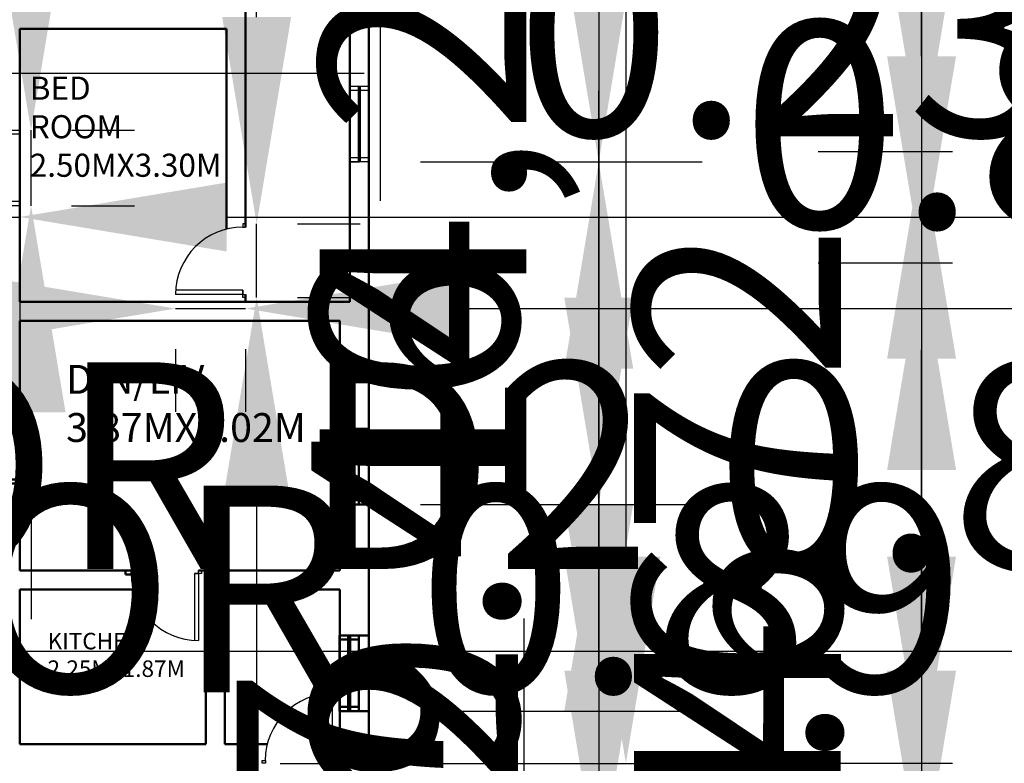
# Model space of a CAD drawing. Units: metres. Extents: x 782 to 1487, y 1262 to 7446.
# Tile 14 of 25: x 828 to 840, y 1293 to 1302. Entities that reach past the tile are written whole.
import ezdxf

# ---------------------------------------------------------------- set-up
doc = ezdxf.new("R2010")
doc.units = ezdxf.units.M
for name, color, linetype, lineweight in [('A-ANNO-DIMS', 2, 'Continuous', 18), ('A-AREA-IDEN', 3, 'Continuous', 18), ('A-DOOR', 4, 'Continuous', 25), ('A-GLAZ', 4, 'Continuous', 25), ('A-WALL', 7, 'Continuous', 50)]:
    doc.layers.add(name, color=color, linetype=linetype, lineweight=lineweight)
doc.styles.get("Standard").update_dxf_attribs({"font": 'arial.ttf'})
doc.dimstyles.new('ISO-25', dxfattribs={"dimtxt": 2.5, "dimasz": 2.5, "dimexe": 1.25, "dimexo": 0.625, "dimtad": 1, "dimtxsty": 'Standard', "dimcen": 2.5, "dimadec": 0, "dimazin": 0, "dimtfac": 1, "dimtmove": 0, "dimatfit": 3, "dimfxl": 1, "dimarcsym": 0})

# ---------------------------------------------------------------- blocks, each defined once
blk = doc.blocks.new('*D6')
at = {"layer": 'A-ANNO-DIMS', "color": 0, "lineweight": -2, "transparency": 16777216}
for p, q in [((833.037, 1307.327), (836.768, 1307.327)), ((835.518, 1304.827), (835.518, 1295.567)), ((833.037, 1293.067), (836.768, 1293.067))]:
    blk.add_line(p, q, dxfattribs=at)
at = {"layer": 'A-ANNO-DIMS', "color": 0, "transparency": 16777216}
for points in [[(835.102, 1304.827), (835.935, 1304.827), (835.518, 1307.327)], [(835.102, 1295.567), (835.935, 1295.567), (835.518, 1293.067)]]:
    blk.add_solid(points, dxfattribs=at)
at = {"layer": 'Defpoints', "color": 0, "transparency": 16777216}
for p in [(832.412, 1307.327), (832.412, 1293.067), (835.518, 1293.067)]:
    blk.add_point(p, dxfattribs=at)
at = {"layer": 'A-ANNO-DIMS', "color": 0, "transparency": 16777216, "insert": (833.391, 1300.197), "char_height": 2.5, "attachment_point": 5, "rotation": 90}
blk.add_mtext('14,26', dxfattribs=at)
blk = doc.blocks.new('DOOR-810')
for p, q in [((0.813, 0.089), (0, 0.089)), ((0.813, 0.038), (0.813, 0.089))]:
    blk.add_line(p, q)
for points in [[(0.813, 0.851), (0.846, 0.851), (0.846, 0.89), (0.813, 0.89)], [(0.813, 0.038), (0.847, 0.038), (0.847, 0), (0.813, 0)]]:
    blk.add_lwpolyline(points, close=True)
blk.add_lwpolyline([(0.813, 0.089), (0.813, 0.038), (0, 0.038)])
blk.add_arc((0.813, 0.038), 0.813, 90, 180)
blk = doc.blocks.new('DOOR-810-B')
for p, q in [((0, 0.813), (0, 0.846)), ((0.812, 0.813), (0.762, 0.813)), ((0.762, 0.813), (0.762, 0))]:
    blk.add_line(p, q)
blk.add_lwpolyline([(0.812, 0.813), (0.812, 0.846), (0.85, 0.846), (0.85, 0.813)], close=True)
blk.add_lwpolyline([(0.762, 0.813), (0.812, 0.813), (0.812, 0)])
blk.add_arc((0.812, 0.813), 0.813, 180, 270)
blk = doc.blocks.new('DOOR-810-C')
for p, q in [((0.801, 0.034), (0.801, 0.847)), ((0.851, 0.034), (0.801, 0.034))]:
    blk.add_line(p, q)
blk.add_lwpolyline([(0.801, 0.034), (0.851, 0.034), (0.851, 0.847)])
for points in [[(0.039, 0.034), (0.039, 0.002), (0, 0.002), (0, 0.034)], [(0.851, 0.034), (0.851, 0), (0.889, 0), (0.889, 0.034)]]:
    blk.add_lwpolyline(points, close=True)
blk.add_arc((0.851, 0.034), 0.813, 90, 180)
blk = doc.blocks.new('WIN-900')
for p, q in [((0, 0), (0, 0.914)), ((0, 0.914), (0.23, 0.914)), ((0.23, 0.863), (0, 0.863)), ((0.102, 0), (0.102, 0.914)), ((0.115, 0), (0.115, 0.914)), ((0.128, 0), (0.128, 0.914)), ((0.23, 0.914), (0.23, 0)), ((0.23, 0.914), (0.23, 0.863)), ((0.23, 0.051), (0, 0.051)), ((0.23, 0), (0.23, 0.051)), ((0.23, 0), (0, 0)), ((0, 0), (0.115, 0))]:
    blk.add_line(p, q)
blk = doc.blocks.new('*D20')
at = {"layer": 'A-ANNO-DIMS', "color": 0, "lineweight": -2, "transparency": 16777216}
for p, q in [((831.056, 1302.088), (831.056, 1337.678)), ((831.056, 1298.698), (831.056, 1299.588)), ((831.548, 1299.588), (832.306, 1299.588)), ((831.548, 1298.698), (832.306, 1298.698)), ((831.056, 1296.198), (831.056, 1293.698))]:
    blk.add_line(p, q, dxfattribs=at)
at = {"layer": 'A-ANNO-DIMS', "color": 0, "transparency": 16777216}
for points in [[(830.64, 1302.088), (831.473, 1302.088), (831.056, 1299.588)], [(830.64, 1296.198), (831.473, 1296.198), (831.056, 1298.698)]]:
    blk.add_solid(points, dxfattribs=at)
at = {"layer": 'Defpoints', "color": 0, "transparency": 16777216}
for p in [(830.923, 1299.588), (831.056, 1299.588), (830.923, 1298.698)]:
    blk.add_point(p, dxfattribs=at)
at = {"layer": 'A-ANNO-DIMS', "color": 0, "transparency": 16777216, "insert": (829.138, 1321.133), "char_height": 2.5, "attachment_point": 5, "rotation": 90}
blk.add_mtext('DOOR D1 0.89 TYP.', dxfattribs=at)
blk = doc.blocks.new('*D21')
at = {"layer": 'A-ANNO-DIMS', "color": 0, "lineweight": -2, "transparency": 16777216}
for p, q in [((827.576, 1298.565), (825.076, 1298.565)), ((830.076, 1298.565), (830.923, 1298.565)), ((833.423, 1298.565), (852.255, 1298.565)), ((830.076, 1298.073), (830.076, 1297.315)), ((830.923, 1298.073), (830.923, 1297.315))]:
    blk.add_line(p, q, dxfattribs=at)
at = {"layer": 'A-ANNO-DIMS', "color": 0, "transparency": 16777216}
for points in [[(827.576, 1298.981), (827.576, 1298.148), (830.076, 1298.565)], [(833.423, 1298.981), (833.423, 1298.148), (830.923, 1298.565)]]:
    blk.add_solid(points, dxfattribs=at)
at = {"layer": 'Defpoints', "color": 0, "transparency": 16777216}
for p in [(830.076, 1298.698), (830.923, 1298.698), (830.923, 1298.565)]:
    blk.add_point(p, dxfattribs=at)
at = {"layer": 'A-ANNO-DIMS', "color": 0, "transparency": 16777216, "insert": (844.089, 1300.466), "char_height": 2.5, "attachment_point": 5}
blk.add_mtext('0.85 TYP.', dxfattribs=at)
blk = doc.blocks.new('*D22')
at = {"layer": 'A-ANNO-DIMS', "color": 0, "lineweight": -2, "transparency": 16777216}
for p, q in [((812.79, 1292.934), (810.29, 1292.934)), ((815.29, 1292.934), (816.179, 1292.934)), ((818.679, 1292.934), (848.834, 1292.934)), ((815.29, 1292.442), (815.29, 1291.684)), ((816.179, 1292.442), (816.179, 1291.684))]:
    blk.add_line(p, q, dxfattribs=at)
at = {"layer": 'A-ANNO-DIMS', "color": 0, "transparency": 16777216}
for points in [[(812.79, 1293.351), (812.79, 1292.517), (815.29, 1292.934)], [(818.679, 1293.351), (818.679, 1292.517), (816.179, 1292.934)]]:
    blk.add_solid(points, dxfattribs=at)
at = {"layer": 'Defpoints', "color": 0, "transparency": 16777216}
for p in [(815.29, 1293.067), (816.179, 1293.067), (816.179, 1292.934)]:
    blk.add_point(p, dxfattribs=at)
at = {"layer": 'A-ANNO-DIMS', "color": 0, "transparency": 16777216, "insert": (835.007, 1294.852), "char_height": 2.5, "attachment_point": 5}
blk.add_mtext('DOOR 0.89 TYP.', dxfattribs=at)
blk = doc.blocks.new('*D24')
at = {"layer": 'A-ANNO-DIMS', "color": 0, "lineweight": -2, "transparency": 16777216}
for p, q in [((811.209, 1294.423), (808.709, 1294.423)), ((813.709, 1294.423), (814.559, 1294.423)), ((817.059, 1294.423), (852.649, 1294.423)), ((813.709, 1293.926), (813.709, 1293.173)), ((814.559, 1293.926), (814.559, 1293.173))]:
    blk.add_line(p, q, dxfattribs=at)
at = {"layer": 'A-ANNO-DIMS', "color": 0, "transparency": 16777216}
for points in [[(811.209, 1294.84), (811.209, 1294.006), (813.709, 1294.423)], [(817.059, 1294.84), (817.059, 1294.006), (814.559, 1294.423)]]:
    blk.add_solid(points, dxfattribs=at)
at = {"layer": 'Defpoints', "color": 0, "transparency": 16777216}
for p in [(813.709, 1294.551), (814.559, 1294.551), (814.559, 1294.423)]:
    blk.add_point(p, dxfattribs=at)
at = {"layer": 'A-ANNO-DIMS', "color": 0, "transparency": 16777216, "insert": (836.104, 1296.342), "char_height": 2.5, "attachment_point": 5}
blk.add_mtext('DOOR D2 0.85 TYP.', dxfattribs=at)
blk = doc.blocks.new('*D26')
at = {"layer": 'A-ANNO-DIMS', "color": 0, "lineweight": -2, "transparency": 16777216}
for p, q in [((828.33, 1303.223), (828.33, 1342.718)), ((828.33, 1299.809), (828.33, 1300.723)), ((828.818, 1300.723), (829.58, 1300.723)), ((828.818, 1299.809), (829.58, 1299.809)), ((828.33, 1297.309), (828.33, 1294.809))]:
    blk.add_line(p, q, dxfattribs=at)
at = {"layer": 'A-ANNO-DIMS', "color": 0, "transparency": 16777216}
for points in [[(827.913, 1303.223), (828.747, 1303.223), (828.33, 1300.723)], [(827.913, 1297.309), (828.747, 1297.309), (828.33, 1299.809)]]:
    blk.add_solid(points, dxfattribs=at)
at = {"layer": 'Defpoints', "color": 0, "transparency": 16777216}
for p in [(828.193, 1300.723), (828.33, 1300.723), (828.193, 1299.809)]:
    blk.add_point(p, dxfattribs=at)
at = {"layer": 'A-ANNO-DIMS', "color": 0, "transparency": 16777216, "insert": (826.412, 1324.22), "char_height": 2.5, "attachment_point": 5, "rotation": 90}
blk.add_mtext('WINDOW W 0.91 TYP.', dxfattribs=at)
blk = doc.blocks.new('*D27')
at = {"layer": 'A-ANNO-DIMS', "color": 0, "lineweight": -2, "transparency": 16777216}
for p, q in [((825.463, 1299.672), (822.963, 1299.672)), ((827.963, 1299.672), (828.193, 1299.672)), ((830.693, 1299.672), (849.525, 1299.672)), ((827.963, 1299.184), (827.963, 1298.422)), ((828.193, 1299.184), (828.193, 1298.422))]:
    blk.add_line(p, q, dxfattribs=at)
at = {"layer": 'A-ANNO-DIMS', "color": 0, "transparency": 16777216}
for points in [[(825.463, 1300.088), (825.463, 1299.255), (827.963, 1299.672)], [(830.693, 1300.088), (830.693, 1299.255), (828.193, 1299.672)]]:
    blk.add_solid(points, dxfattribs=at)
at = {"layer": 'Defpoints', "color": 0, "transparency": 16777216}
for p in [(827.963, 1299.809), (828.193, 1299.809), (828.193, 1299.672)]:
    blk.add_point(p, dxfattribs=at)
at = {"layer": 'A-ANNO-DIMS', "color": 0, "transparency": 16777216, "insert": (841.359, 1301.574), "char_height": 2.5, "attachment_point": 5}
blk.add_mtext('0.23 TYP.', dxfattribs=at)
blk = doc.blocks.new('*D28')
at = {"layer": 'A-ANNO-DIMS', "color": 0, "lineweight": -2, "transparency": 16777216}
for p, q in [((832.55, 1308.281), (832.55, 1349.718)), ((832.55, 1304.867), (832.55, 1305.781)), ((833.038, 1305.781), (833.8, 1305.781)), ((833.038, 1304.867), (833.8, 1304.867)), ((832.55, 1302.367), (832.55, 1299.867))]:
    blk.add_line(p, q, dxfattribs=at)
at = {"layer": 'A-ANNO-DIMS', "color": 0, "transparency": 16777216}
for points in [[(832.134, 1308.281), (832.967, 1308.281), (832.55, 1305.781)], [(832.134, 1302.367), (832.967, 1302.367), (832.55, 1304.867)]]:
    blk.add_solid(points, dxfattribs=at)
at = {"layer": 'Defpoints', "color": 0, "transparency": 16777216}
for p in [(832.413, 1305.781), (832.55, 1305.781), (832.413, 1304.867)]:
    blk.add_point(p, dxfattribs=at)
at = {"layer": 'A-ANNO-DIMS', "color": 0, "transparency": 16777216, "insert": (830.632, 1330.25), "char_height": 2.5, "attachment_point": 5, "rotation": 90}
blk.add_mtext('WINDOW W1 0.91 TYP.', dxfattribs=at)
blk = doc.blocks.new('*D30')
at = {"layer": 'A-ANNO-DIMS', "color": 0, "lineweight": -2, "transparency": 16777216}
for p, q in [((792.059, 1301.411), (789.559, 1301.411)), ((794.559, 1301.411), (794.946, 1301.411)), ((797.446, 1301.411), (832.354, 1301.411)), ((794.559, 1300.844), (794.559, 1300.161)), ((794.946, 1300.844), (794.946, 1300.161))]:
    blk.add_line(p, q, dxfattribs=at)
at = {"layer": 'A-ANNO-DIMS', "color": 0, "transparency": 16777216}
for points in [[(792.059, 1301.827), (792.059, 1300.994), (794.559, 1301.411)], [(797.446, 1301.827), (797.446, 1300.994), (794.946, 1301.411)]]:
    blk.add_solid(points, dxfattribs=at)
at = {"layer": 'Defpoints', "color": 0, "transparency": 16777216}
for p in [(794.559, 1301.469), (794.946, 1301.469), (794.946, 1301.411)]:
    blk.add_point(p, dxfattribs=at)
at = {"layer": 'A-ANNO-DIMS', "color": 0, "transparency": 16777216, "insert": (816.15, 1303.33), "char_height": 2.5, "attachment_point": 5}
blk.add_mtext('COLUMN 0.39 TYP.', dxfattribs=at)
blk = doc.blocks.new('*D87')
at = {"layer": 'A-ANNO-DIMS', "color": 0, "lineweight": -2, "transparency": 16777216}
for p, q in [((835.19, 1309.827), (835.19, 1312.327)), ((833.037, 1307.327), (836.44, 1307.327)), ((835.19, 1307.327), (835.19, 1304.867)), ((833.038, 1304.867), (836.44, 1304.867)), ((835.19, 1302.367), (835.19, 1292.082))]:
    blk.add_line(p, q, dxfattribs=at)
at = {"layer": 'A-ANNO-DIMS', "color": 0, "transparency": 16777216}
for points in [[(834.774, 1309.827), (835.607, 1309.827), (835.19, 1307.327)], [(834.774, 1302.367), (835.607, 1302.367), (835.19, 1304.867)]]:
    blk.add_solid(points, dxfattribs=at)
at = {"layer": 'Defpoints', "color": 0, "transparency": 16777216}
for p in [(832.412, 1307.327), (832.413, 1304.867), (835.19, 1304.867)]:
    blk.add_point(p, dxfattribs=at)
at = {"layer": 'A-ANNO-DIMS', "color": 0, "transparency": 16777216, "insert": (833.289, 1295.974), "char_height": 2.5, "attachment_point": 5, "rotation": 90}
blk.add_mtext('2.46', dxfattribs=at)
blk = doc.blocks.new('*D88')
at = {"layer": 'A-ANNO-DIMS', "color": 0, "lineweight": -2, "transparency": 16777216}
for p, q in [((835.19, 1307.367), (835.19, 1309.867)), ((833.038, 1304.867), (836.44, 1304.867)), ((835.19, 1304.867), (835.19, 1300.338)), ((833.038, 1300.338), (836.44, 1300.338)), ((835.19, 1297.838), (835.19, 1285.546))]:
    blk.add_line(p, q, dxfattribs=at)
at = {"layer": 'A-ANNO-DIMS', "color": 0, "transparency": 16777216}
for points in [[(834.774, 1307.367), (835.607, 1307.367), (835.19, 1304.867)], [(834.774, 1297.838), (835.607, 1297.838), (835.19, 1300.338)]]:
    blk.add_solid(points, dxfattribs=at)
at = {"layer": 'Defpoints', "color": 0, "transparency": 16777216}
for p in [(832.413, 1304.867), (832.413, 1300.338), (835.19, 1300.338)]:
    blk.add_point(p, dxfattribs=at)
at = {"layer": 'A-ANNO-DIMS', "color": 0, "transparency": 16777216, "insert": (833.289, 1290.442), "char_height": 2.5, "attachment_point": 5, "rotation": 90}
blk.add_mtext('4.529', dxfattribs=at)
blk = doc.blocks.new('*D89')
at = {"layer": 'A-ANNO-DIMS', "color": 0, "lineweight": -2, "transparency": 16777216}
for p, q in [((835.19, 1302.838), (835.19, 1305.338)), ((833.038, 1300.338), (836.44, 1300.338)), ((835.19, 1300.338), (835.19, 1296.196)), ((833.037, 1296.196), (836.44, 1296.196)), ((835.19, 1293.696), (835.19, 1281.435))]:
    blk.add_line(p, q, dxfattribs=at)
at = {"layer": 'A-ANNO-DIMS', "color": 0, "transparency": 16777216}
for points in [[(834.774, 1302.838), (835.607, 1302.838), (835.19, 1300.338)], [(834.774, 1293.696), (835.607, 1293.696), (835.19, 1296.196)]]:
    blk.add_solid(points, dxfattribs=at)
at = {"layer": 'Defpoints', "color": 0, "transparency": 16777216}
for p in [(832.413, 1300.338), (832.412, 1296.196), (835.19, 1296.196)]:
    blk.add_point(p, dxfattribs=at)
at = {"layer": 'A-ANNO-DIMS', "color": 0, "transparency": 16777216, "insert": (833.31, 1286.315), "char_height": 2.5, "attachment_point": 5, "rotation": 90}
blk.add_mtext('4.142', dxfattribs=at)
blk = doc.blocks.new('*D90')
at = {"layer": 'A-ANNO-DIMS', "color": 0, "lineweight": -2, "transparency": 16777216}
for p, q in [((835.19, 1298.696), (835.19, 1301.196)), ((833.037, 1296.196), (836.44, 1296.196)), ((835.19, 1296.196), (835.19, 1293.699)), ((833.037, 1293.699), (836.44, 1293.699)), ((835.19, 1291.199), (835.19, 1280.921))]:
    blk.add_line(p, q, dxfattribs=at)
at = {"layer": 'A-ANNO-DIMS', "color": 0, "transparency": 16777216}
for points in [[(834.774, 1298.696), (835.607, 1298.696), (835.19, 1296.196)], [(834.774, 1291.199), (835.607, 1291.199), (835.19, 1293.699)]]:
    blk.add_solid(points, dxfattribs=at)
at = {"layer": 'Defpoints', "color": 0, "transparency": 16777216}
for p in [(832.412, 1296.196), (832.412, 1293.699), (835.19, 1293.699)]:
    blk.add_point(p, dxfattribs=at)
at = {"layer": 'A-ANNO-DIMS', "color": 0, "transparency": 16777216, "insert": (833.289, 1284.81), "char_height": 2.5, "attachment_point": 5, "rotation": 90}
blk.add_mtext('2.50', dxfattribs=at)
blk = doc.blocks.new('*D91')
at = {"layer": 'A-ANNO-DIMS', "color": 0, "lineweight": -2, "transparency": 16777216}
for p, q in [((835.19, 1296.199), (835.19, 1298.699)), ((833.037, 1293.699), (836.44, 1293.699)), ((835.19, 1293.699), (835.19, 1293.067)), ((833.037, 1293.067), (836.44, 1293.067)), ((835.19, 1290.567), (835.19, 1278.407))]:
    blk.add_line(p, q, dxfattribs=at)
at = {"layer": 'A-ANNO-DIMS', "color": 0, "transparency": 16777216}
for points in [[(834.774, 1296.199), (835.607, 1296.199), (835.19, 1293.699)], [(834.774, 1290.567), (835.607, 1290.567), (835.19, 1293.067)]]:
    blk.add_solid(points, dxfattribs=at)
at = {"layer": 'Defpoints', "color": 0, "transparency": 16777216}
for p in [(832.412, 1293.699), (832.412, 1293.067), (835.19, 1293.067)]:
    blk.add_point(p, dxfattribs=at)
at = {"layer": 'A-ANNO-DIMS', "color": 0, "transparency": 16777216, "insert": (833.288, 1283.237), "char_height": 2.5, "attachment_point": 5, "rotation": 90}
blk.add_mtext('0.632', dxfattribs=at)
blk = doc.blocks.new('*D92')
at = {"layer": 'A-ANNO-DIMS', "color": 0, "lineweight": -2, "transparency": 16777216}
for p, q in [((835.19, 1295.567), (835.19, 1298.067)), ((831.341, 1293.067), (836.44, 1293.067)), ((835.19, 1293.067), (835.19, 1291.686)), ((831.341, 1291.686), (836.44, 1291.686)), ((835.19, 1289.186), (835.19, 1277.718))]:
    blk.add_line(p, q, dxfattribs=at)
at = {"layer": 'A-ANNO-DIMS', "color": 0, "transparency": 16777216}
for points in [[(834.774, 1295.567), (835.607, 1295.567), (835.19, 1293.067)], [(834.774, 1289.186), (835.607, 1289.186), (835.19, 1291.686)]]:
    blk.add_solid(points, dxfattribs=at)
at = {"layer": 'Defpoints', "color": 0, "transparency": 16777216}
for p in [(830.716, 1293.067), (830.716, 1291.686), (835.19, 1291.686)]:
    blk.add_point(p, dxfattribs=at)
at = {"layer": 'A-ANNO-DIMS', "color": 0, "transparency": 16777216, "insert": (833.288, 1282.202), "char_height": 2.5, "attachment_point": 5, "rotation": 90}
blk.add_mtext('1.381', dxfattribs=at)
blk = doc.blocks.new('*D93')
at = {"layer": 'A-ANNO-DIMS', "color": 0, "lineweight": -2, "transparency": 16777216}
for p, q in [((835.19, 1294.186), (835.19, 1296.686)), ((831.341, 1291.686), (836.44, 1291.686)), ((835.19, 1291.686), (835.19, 1290.305)), ((831.341, 1290.305), (836.44, 1290.305)), ((835.19, 1287.805), (835.19, 1276.337))]:
    blk.add_line(p, q, dxfattribs=at)
at = {"layer": 'A-ANNO-DIMS', "color": 0, "transparency": 16777216}
for points in [[(834.774, 1294.186), (835.607, 1294.186), (835.19, 1291.686)], [(834.774, 1287.805), (835.607, 1287.805), (835.19, 1290.305)]]:
    blk.add_solid(points, dxfattribs=at)
at = {"layer": 'Defpoints', "color": 0, "transparency": 16777216}
for p in [(830.716, 1291.686), (830.716, 1290.305), (835.19, 1290.305)]:
    blk.add_point(p, dxfattribs=at)
at = {"layer": 'A-ANNO-DIMS', "color": 0, "transparency": 16777216, "insert": (833.288, 1280.821), "char_height": 2.5, "attachment_point": 5, "rotation": 90}
blk.add_mtext('1.381', dxfattribs=at)
blk = doc.blocks.new('*D109')
at = {"layer": 'A-ANNO-DIMS', "color": 0, "lineweight": -2, "transparency": 16777216}
for p, q in [((839.091, 1308.335), (839.091, 1310.835)), ((839.466, 1305.835), (837.841, 1305.835)), ((839.091, 1305.835), (839.091, 1305.163)), ((839.466, 1305.163), (837.841, 1305.163)), ((839.091, 1302.663), (839.091, 1290.503))]:
    blk.add_line(p, q, dxfattribs=at)
at = {"layer": 'A-ANNO-DIMS', "color": 0, "transparency": 16777216}
for points in [[(838.675, 1308.335), (839.508, 1308.335), (839.091, 1305.835)], [(838.675, 1302.663), (839.508, 1302.663), (839.091, 1305.163)]]:
    blk.add_solid(points, dxfattribs=at)
at = {"layer": 'Defpoints', "color": 0, "transparency": 16777216}
for p in [(840.091, 1305.835), (839.091, 1305.163), (840.091, 1305.163)]:
    blk.add_point(p, dxfattribs=at)
at = {"layer": 'A-ANNO-DIMS', "color": 0, "transparency": 16777216, "insert": (837.19, 1295.333), "char_height": 2.5, "attachment_point": 5, "rotation": 90}
blk.add_mtext('0.672', dxfattribs=at)
blk = doc.blocks.new('*D110')
at = {"layer": 'A-ANNO-DIMS', "color": 0, "lineweight": -2, "transparency": 16777216}
for p, q in [((839.091, 1307.663), (839.091, 1310.163)), ((839.466, 1305.163), (837.841, 1305.163)), ((839.091, 1305.163), (839.091, 1300.459)), ((839.466, 1300.459), (837.841, 1300.459)), ((839.091, 1297.959), (839.091, 1285.683))]:
    blk.add_line(p, q, dxfattribs=at)
at = {"layer": 'A-ANNO-DIMS', "color": 0, "transparency": 16777216}
for points in [[(838.675, 1307.663), (839.508, 1307.663), (839.091, 1305.163)], [(838.675, 1297.959), (839.508, 1297.959), (839.091, 1300.459)]]:
    blk.add_solid(points, dxfattribs=at)
at = {"layer": 'Defpoints', "color": 0, "transparency": 16777216}
for p in [(840.091, 1305.163), (839.091, 1300.459), (840.091, 1300.459)]:
    blk.add_point(p, dxfattribs=at)
at = {"layer": 'A-ANNO-DIMS', "color": 0, "transparency": 16777216, "insert": (837.19, 1290.571), "char_height": 2.5, "attachment_point": 5, "rotation": 90}
blk.add_mtext('4.704', dxfattribs=at)
blk = doc.blocks.new('*D111')
at = {"layer": 'A-ANNO-DIMS', "color": 0, "lineweight": -2, "transparency": 16777216}
for p, q in [((839.091, 1302.959), (839.091, 1305.459)), ((839.466, 1300.459), (837.841, 1300.459)), ((839.091, 1300.459), (839.091, 1299.115)), ((839.466, 1299.115), (837.841, 1299.115)), ((839.091, 1296.615), (839.091, 1284.675))]:
    blk.add_line(p, q, dxfattribs=at)
at = {"layer": 'A-ANNO-DIMS', "color": 0, "transparency": 16777216}
for points in [[(838.675, 1302.959), (839.508, 1302.959), (839.091, 1300.459)], [(838.675, 1296.615), (839.508, 1296.615), (839.091, 1299.115)]]:
    blk.add_solid(points, dxfattribs=at)
at = {"layer": 'Defpoints', "color": 0, "transparency": 16777216}
for p in [(840.091, 1300.459), (839.091, 1299.115), (840.091, 1299.115)]:
    blk.add_point(p, dxfattribs=at)
at = {"layer": 'A-ANNO-DIMS', "color": 0, "transparency": 16777216, "insert": (837.189, 1289.395), "char_height": 2.5, "attachment_point": 5, "rotation": 90}
blk.add_mtext('1.344', dxfattribs=at)
blk = doc.blocks.new('*D112')
at = {"layer": 'A-ANNO-DIMS', "color": 0, "lineweight": -2, "transparency": 16777216}
for p, q in [((839.091, 1301.615), (839.091, 1304.115)), ((839.466, 1299.115), (837.841, 1299.115)), ((839.091, 1299.115), (839.091, 1293.067)), ((839.466, 1293.067), (837.841, 1293.067)), ((839.091, 1290.567), (839.091, 1278.362))]:
    blk.add_line(p, q, dxfattribs=at)
at = {"layer": 'A-ANNO-DIMS', "color": 0, "transparency": 16777216}
for points in [[(838.675, 1301.615), (839.508, 1301.615), (839.091, 1299.115)], [(838.675, 1290.567), (839.508, 1290.567), (839.091, 1293.067)]]:
    blk.add_solid(points, dxfattribs=at)
at = {"layer": 'Defpoints', "color": 0, "transparency": 16777216}
for p in [(840.091, 1299.115), (839.091, 1293.067), (840.091, 1293.067)]:
    blk.add_point(p, dxfattribs=at)
at = {"layer": 'A-ANNO-DIMS', "color": 0, "transparency": 16777216, "insert": (837.19, 1283.215), "char_height": 2.5, "attachment_point": 5, "rotation": 90}
blk.add_mtext('6.048', dxfattribs=at)
blk = doc.blocks.new('*D113')
at = {"layer": 'A-ANNO-DIMS', "color": 0, "lineweight": -2, "transparency": 16777216}
for p, q in [((839.091, 1295.567), (839.091, 1298.067)), ((839.466, 1293.067), (837.841, 1293.067)), ((839.091, 1293.067), (839.091, 1291.686)), ((839.466, 1291.686), (837.841, 1291.686)), ((839.091, 1289.186), (839.091, 1277.718))]:
    blk.add_line(p, q, dxfattribs=at)
at = {"layer": 'A-ANNO-DIMS', "color": 0, "transparency": 16777216}
for points in [[(838.675, 1295.567), (839.508, 1295.567), (839.091, 1293.067)], [(838.675, 1289.186), (839.508, 1289.186), (839.091, 1291.686)]]:
    blk.add_solid(points, dxfattribs=at)
at = {"layer": 'Defpoints', "color": 0, "transparency": 16777216}
for p in [(840.091, 1293.067), (839.091, 1291.686), (840.091, 1291.686)]:
    blk.add_point(p, dxfattribs=at)
at = {"layer": 'A-ANNO-DIMS', "color": 0, "transparency": 16777216, "insert": (837.189, 1282.202), "char_height": 2.5, "attachment_point": 5, "rotation": 90}
blk.add_mtext('1.381', dxfattribs=at)
blk = doc.blocks.new('*D114')
at = {"layer": 'A-ANNO-DIMS', "color": 0, "lineweight": -2, "transparency": 16777216}
for p, q in [((839.091, 1294.186), (839.091, 1296.686)), ((839.466, 1291.686), (837.841, 1291.686)), ((839.091, 1291.686), (839.091, 1290.305)), ((839.466, 1290.305), (837.841, 1290.305)), ((839.091, 1287.805), (839.091, 1276.337))]:
    blk.add_line(p, q, dxfattribs=at)
at = {"layer": 'A-ANNO-DIMS', "color": 0, "transparency": 16777216}
for points in [[(838.675, 1294.186), (839.508, 1294.186), (839.091, 1291.686)], [(838.675, 1287.805), (839.508, 1287.805), (839.091, 1290.305)]]:
    blk.add_solid(points, dxfattribs=at)
at = {"layer": 'Defpoints', "color": 0, "transparency": 16777216}
for p in [(840.091, 1291.686), (839.091, 1290.305), (840.091, 1290.305)]:
    blk.add_point(p, dxfattribs=at)
at = {"layer": 'A-ANNO-DIMS', "color": 0, "transparency": 16777216, "insert": (837.189, 1280.821), "char_height": 2.5, "attachment_point": 5, "rotation": 90}
blk.add_mtext('1.381', dxfattribs=at)
blk = doc.blocks.new('*D157')
at = {"layer": 'A-ANNO-DIMS', "color": 0, "lineweight": -2, "transparency": 16777216}
for p, q in [((834.289, 1282.619), (834.289, 1294.819)), ((835.878, 1282.619), (833.039, 1282.619)), ((834.289, 1278.702), (834.289, 1280.119)), ((835.878, 1276.202), (833.039, 1276.202))]:
    blk.add_line(p, q, dxfattribs=at)
at = {"layer": 'A-ANNO-DIMS', "color": 0, "transparency": 16777216}
for points in [[(833.872, 1280.119), (834.705, 1280.119), (834.289, 1282.619)], [(833.872, 1278.702), (834.705, 1278.702), (834.289, 1276.202)]]:
    blk.add_solid(points, dxfattribs=at)
at = {"layer": 'Defpoints', "color": 0, "transparency": 16777216}
for p in [(834.289, 1282.619), (836.503, 1282.619), (836.503, 1276.202)]:
    blk.add_point(p, dxfattribs=at)
at = {"layer": 'A-ANNO-DIMS', "color": 0, "transparency": 16777216, "insert": (832.387, 1289.969), "char_height": 2.5, "attachment_point": 5, "rotation": 90}
blk.add_mtext('6.417', dxfattribs=at)

msp = doc.modelspace()

# ---------------------------------------------------------------- linework, layer by layer
at = {"layer": 'A-WALL'}
for p, q in [((832.4125, 1303.3374), (832.4125, 1293.0674)), ((832.1825, 1303.1074), (832.1825, 1298.6474)), ((830.9225, 1302.1774), (830.9225, 1299.5481)), ((828.1925, 1298.6474), (828.1925, 1301.9474)), ((828.1925, 1301.9474), (830.6925, 1301.9474)), ((830.6925, 1301.9474), (830.6925, 1299.5248)), ((828.1925, 1298.6474), (832.0625, 1298.6474)), ((830.9225, 1298.736), (830.9225, 1298.6474)), ((830.9225, 1298.6474), (830.9225, 1298.6982)), ((832.1825, 1298.6474), (832.0625, 1298.6474)), ((828.1925, 1295.3974), (828.1925, 1298.4174)), ((828.1925, 1298.4174), (832.0625, 1298.4174)), ((828.1925, 1298.4174), (832.0625, 1298.4174)), ((832.0625, 1298.4174), (832.0625, 1295.3974)), ((827.9641, 1297.3636), (828.1941, 1297.3636)), ((828.1941, 1297.3636), (828.1941, 1296.4496)), ((828.1941, 1297.3636), (828.1941, 1297.3128)), ((828.1941, 1297.3128), (827.9641, 1297.3128)), ((832.0626, 1296.196), (832.0626, 1297.11)), ((832.0626, 1297.11), (832.2926, 1297.11)), ((832.1649, 1296.196), (832.1649, 1297.11)), ((832.1776, 1296.196), (832.1776, 1297.11)), ((832.1903, 1296.196), (832.1903, 1297.11)), ((832.2926, 1297.11), (832.2926, 1296.196)), ((832.2926, 1297.11), (832.2926, 1297.0592)), ((832.2926, 1297.11), (832.4125, 1297.11)), ((832.4125, 1297.11), (832.4125, 1296.196)), ((832.2926, 1297.0592), (832.0626, 1297.0592)), ((828.1941, 1296.5004), (827.9641, 1296.5004)), ((828.1941, 1296.4496), (828.1941, 1296.5004)), ((828.1941, 1296.4496), (827.9641, 1296.4496)), ((832.2926, 1296.2468), (832.0626, 1296.2468)), ((832.2926, 1296.196), (832.0626, 1296.196)), ((832.0626, 1296.196), (832.1776, 1296.196)), ((832.2926, 1296.196), (832.2926, 1296.2468)), ((832.4125, 1296.196), (832.2926, 1296.196)), ((829.5418, 1295.3974), (828.1925, 1295.3974)), ((829.5418, 1295.3974), (828.1925, 1295.3974)), ((829.541, 1295.3974), (829.4731, 1295.3974)), ((829.4731, 1295.3974), (829.4731, 1295.3502)), ((829.4731, 1295.3502), (829.5412, 1295.3502)), ((830.4425, 1295.3974), (830.3538, 1295.3974)), ((832.0625, 1295.3974), (830.3538, 1295.3974)), ((830.4425, 1295.3974), (830.3917, 1295.3974)), ((830.4425, 1295.1674), (830.4425, 1295.3974)), ((829.5651, 1295.1674), (828.1925, 1295.1674)), ((828.1925, 1295.1674), (828.1925, 1293.2974)), ((829.5651, 1295.1674), (828.1925, 1295.1674)), ((830.4425, 1293.2974), (830.4425, 1295.1674)), ((832.0625, 1295.1674), (830.4425, 1295.1674)), ((830.6725, 1293.2974), (830.6725, 1295.1674)), ((832.0625, 1293.2974), (832.0625, 1295.1674)), ((832.0592, 1293.6994), (832.0592, 1294.6134)), ((832.0592, 1294.6134), (832.2892, 1294.6134)), ((832.1615, 1293.6994), (832.1615, 1294.6134)), ((832.1742, 1293.6994), (832.1742, 1294.6134)), ((832.1869, 1293.6994), (832.1869, 1294.6134)), ((832.2892, 1294.6134), (832.2892, 1293.6994)), ((832.2892, 1294.6134), (832.2892, 1294.5626)), ((832.2892, 1294.6134), (832.4125, 1294.6134)), ((832.4125, 1294.6134), (832.4125, 1293.6994)), ((832.2892, 1294.5626), (832.0592, 1294.5626)), ((832.2892, 1293.7502), (832.0592, 1293.7502)), ((832.2892, 1293.6994), (832.0592, 1293.6994)), ((832.0592, 1293.6994), (832.1742, 1293.6994)), ((832.2892, 1293.6994), (832.2892, 1293.7502)), ((832.4125, 1293.6994), (832.2892, 1293.6994)), ((828.1925, 1293.2974), (830.4425, 1293.2974)), ((830.6725, 1293.2974), (831.1851, 1293.2974)), ((831.9738, 1293.2974), (832.0625, 1293.2974))]:
    msp.add_line(p, q, dxfattribs=at)

# ---------------------------------------------------------------- block references
at = {"layer": 'A-DOOR'}
for name, p in [('DOOR-810', (830.076, 1298.698)), ('DOOR-810-B', (829.541, 1294.551)), ('DOOR-810-C', (831.122, 1293.067))]:
    msp.add_blockref(name, p, dxfattribs=at)
at = {"layer": 'A-GLAZ'}
for p in [(832.183, 1300.338), (827.963, 1299.809)]:
    msp.add_blockref('WIN-900', p, dxfattribs=at)

# ---------------------------------------------------------------- texts
at = {"layer": 'A-AREA-IDEN', "attachment_point": 1}
for s, width, gutter_width, insert, char_height in [('BED ROOM\\P2.50MX3.30M', 0.64421, 6.9836, (828.3137, 1301.3688), 0.279342), ('DIN/LIV\\P3.87MX3.02M', 0.805163, 8.7284, (828.7531, 1297.8835), 0.349134), ('{\\H0.4x;\\PKITCHEN\\P2.25MX1.87M}', 1.153085, 12.5, (828.5294, 1294.9782), 0.5)]:
    msp.add_mtext_dynamic_manual_height_columns(s, width=width, gutter_width=gutter_width, heights=[0], dxfattribs=dict(at, insert=insert, char_height=char_height))

# ---------------------------------------------------------------- dimensions: what is measured, and where the dimension line sits
at = {"layer": 'A-ANNO-DIMS'}
for base, p1, p2, text, picture, middle in [((832.5503, 1305.7809), (832.4132, 1304.8669), (832.4132, 1305.7809), 'WINDOW W1 <> TYP.', '*D28', (830.6318, 1330.2497)), ((828.3302, 1300.7228), (828.1931, 1299.8088), (828.1931, 1300.7228), 'WINDOW W <> TYP.', '*D26', (826.4117, 1324.2204)), ((831.0564, 1299.5877), (830.923, 1298.6982), (830.923, 1299.5877), 'DOOR D1 <> TYP.', '*D20', (829.138, 1321.1327))]:
    dim = msp.add_linear_dim(base=base, p1=p1, p2=p2, angle=90, text=text, dimstyle='ISO-25', override={"dimdec": 2, "dimlfac": 1, "dimrnd": 0, "dimzin": 0, "dimdsep": 46, "dimlunit": 2}, dxfattribs=at)
    dim.commit()
    dim.dimension.update_dxf_attribs({"geometry": picture, "text_midpoint": middle})
for base, p1, p2, override, picture, middle in [((835.1905, 1304.8669), (832.4125, 1307.3274), (832.4132, 1304.8669), {"dimdec": 2, "dimlfac": 1, "dimrnd": 0, "dimzin": 0, "dimdsep": 46, "dimlunit": 2}, '*D87', (833.289, 1295.9745)), ((839.0913, 1305.1633), (840.0913, 1305.8353), (840.0913, 1305.1633), {"dimdec": 3, "dimlfac": 1, "dimrnd": 0, "dimzin": 0, "dimdsep": 46, "dimlunit": 2}, '*D109', (837.1899, 1295.333)), ((839.0913, 1300.4593), (840.0913, 1305.1633), (840.0913, 1300.4593), {"dimdec": 3, "dimlfac": 1, "dimrnd": 0, "dimzin": 0, "dimdsep": 46, "dimlunit": 2}, '*D110', (837.1899, 1290.571)), ((835.1905, 1300.3378), (832.4132, 1304.8669), (832.4131, 1300.3378), {"dimdec": 3, "dimlfac": 1, "dimrnd": 0, "dimzin": 0, "dimdsep": 46, "dimlunit": 2}, '*D88', (833.289, 1290.4419)), ((835.5183, 1293.0674), (832.4125, 1307.3274), (832.4125, 1293.0674), {"dimclrd": 0, "dimclre": 0, "dimclrt": 0}, '*D6', (833.3909, 1300.1974)), ((839.0913, 1299.1153), (840.0913, 1300.4593), (840.0913, 1299.1153), {"dimdec": 3, "dimlfac": 1, "dimrnd": 0, "dimzin": 0, "dimdsep": 46, "dimlunit": 2}, '*D111', (837.189, 1289.395)), ((835.1905, 1296.196), (832.4131, 1300.3378), (832.4125, 1296.196), {"dimdec": 3, "dimlfac": 1, "dimrnd": 0, "dimzin": 0, "dimdsep": 46, "dimlunit": 2}, '*D89', (833.3103, 1286.3153)), ((839.0913, 1293.0674), (840.0913, 1299.1153), (840.0913, 1293.0674), {"dimdec": 3, "dimlfac": 1, "dimrnd": 0, "dimzin": 0, "dimdsep": 46, "dimlunit": 2}, '*D112', (837.1899, 1283.2149)), ((835.1905, 1293.6994), (832.4125, 1296.196), (832.4125, 1293.6994), {"dimdec": 2, "dimlfac": 1, "dimrnd": 0, "dimzin": 0, "dimdsep": 46, "dimlunit": 2}, '*D90', (833.289, 1284.8104)), ((835.1905, 1293.0674), (832.4125, 1293.6994), (832.4125, 1293.0674), {"dimdec": 3, "dimlfac": 1, "dimrnd": 0, "dimzin": 0, "dimdsep": 46, "dimlunit": 2}, '*D91', (833.2882, 1283.2371)), ((835.1905, 1291.6863), (830.7156, 1293.0674), (830.7156, 1291.6863), {"dimdec": 3, "dimlfac": 1, "dimrnd": 0, "dimzin": 0, "dimdsep": 46, "dimlunit": 2}, '*D92', (833.2882, 1282.2022)), ((839.0913, 1291.6863), (840.0913, 1293.0674), (840.0913, 1291.6863), {"dimdec": 3, "dimlfac": 1, "dimrnd": 0, "dimzin": 0, "dimdsep": 46, "dimlunit": 2}, '*D113', (837.189, 1282.2022)), ((835.1905, 1290.3053), (830.7156, 1291.6863), (830.7156, 1290.3053), {"dimdec": 3, "dimlfac": 1, "dimrnd": 0, "dimzin": 0, "dimdsep": 46, "dimlunit": 2}, '*D93', (833.2882, 1280.8211)), ((839.0913, 1290.3053), (840.0913, 1291.6863), (840.0913, 1290.3053), {"dimdec": 3, "dimlfac": 1, "dimrnd": 0, "dimzin": 0, "dimdsep": 46, "dimlunit": 2}, '*D114', (837.189, 1280.8211)), ((834.2886, 1282.619), (836.5033, 1276.2022), (836.5033, 1282.619), {"dimdec": 3, "dimlfac": 1, "dimrnd": 0, "dimzin": 0, "dimdsep": 46, "dimlunit": 2}, '*D157', (832.3871, 1289.9689))]:
    dim = msp.add_linear_dim(base=base, p1=p1, p2=p2, angle=90, dimstyle='ISO-25', override=override, dxfattribs=at)
    dim.commit()
    dim.dimension.update_dxf_attribs({"geometry": picture, "text_midpoint": middle})
for base, p1, p2, text, picture, middle in [((794.9459, 1301.4107), (794.559, 1301.4687), (794.9459, 1301.4687), 'COLUMN <> TYP.', '*D30', (816.1499, 1303.33)), ((828.1931, 1299.6717), (827.9631, 1299.8088), (828.1931, 1299.8088), '<> TYP.', '*D27', (841.359, 1301.574)), ((814.5592, 1294.4231), (813.7086, 1294.5507), (814.5592, 1294.5507), 'DOOR D2 <> TYP.', '*D24', (836.1042, 1296.3416)), ((830.923, 1298.5648), (830.0763, 1298.6982), (830.923, 1298.6982), '<> TYP.', '*D21', (844.0889, 1300.4662)), ((816.1792, 1292.934), (815.2897, 1293.0674), (816.1792, 1293.0674), 'DOOR <> TYP.', '*D22', (835.0068, 1294.8525))]:
    dim = msp.add_linear_dim(base=base, p1=p1, p2=p2, text=text, dimstyle='ISO-25', override={"dimdec": 2, "dimlfac": 1, "dimrnd": 0, "dimzin": 0, "dimdsep": 46, "dimlunit": 2}, dxfattribs=at)
    dim.commit()
    dim.dimension.update_dxf_attribs({"geometry": picture, "text_midpoint": middle})

doc.saveas('drawing.dxf')
